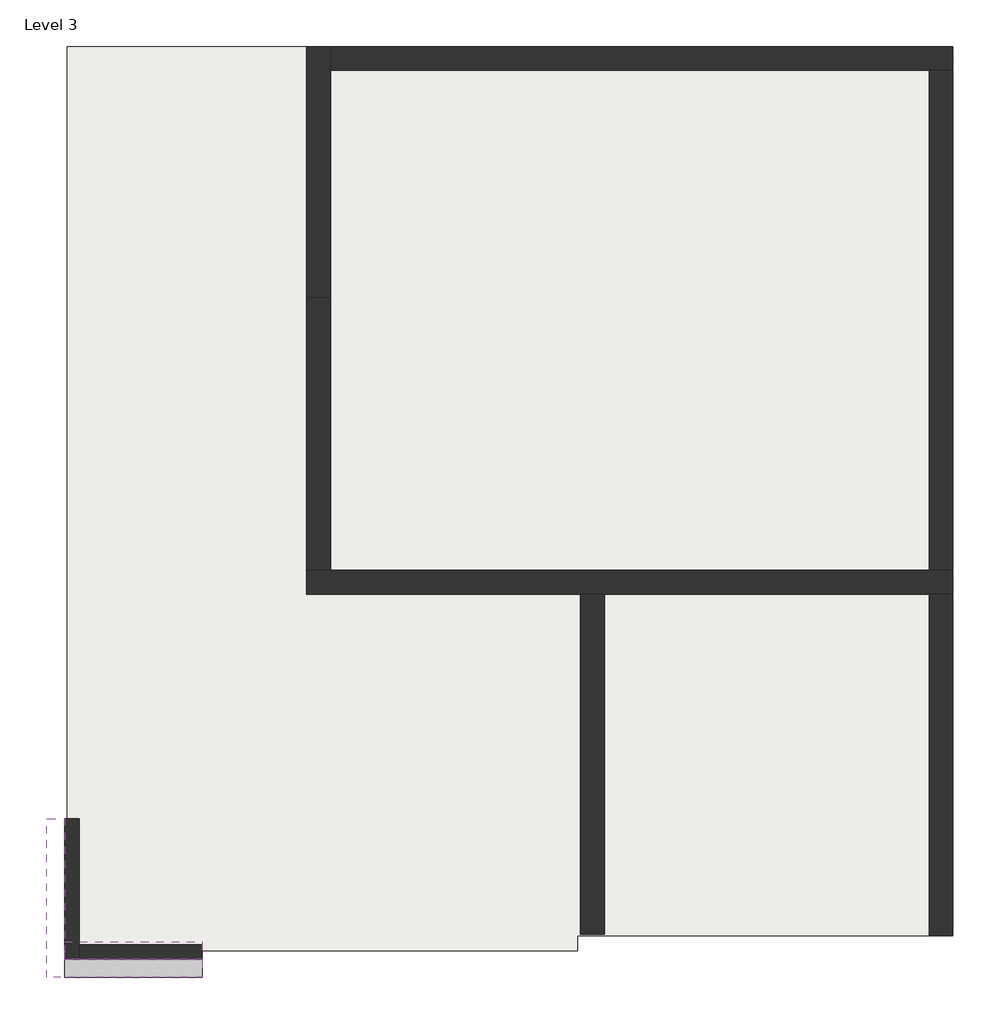
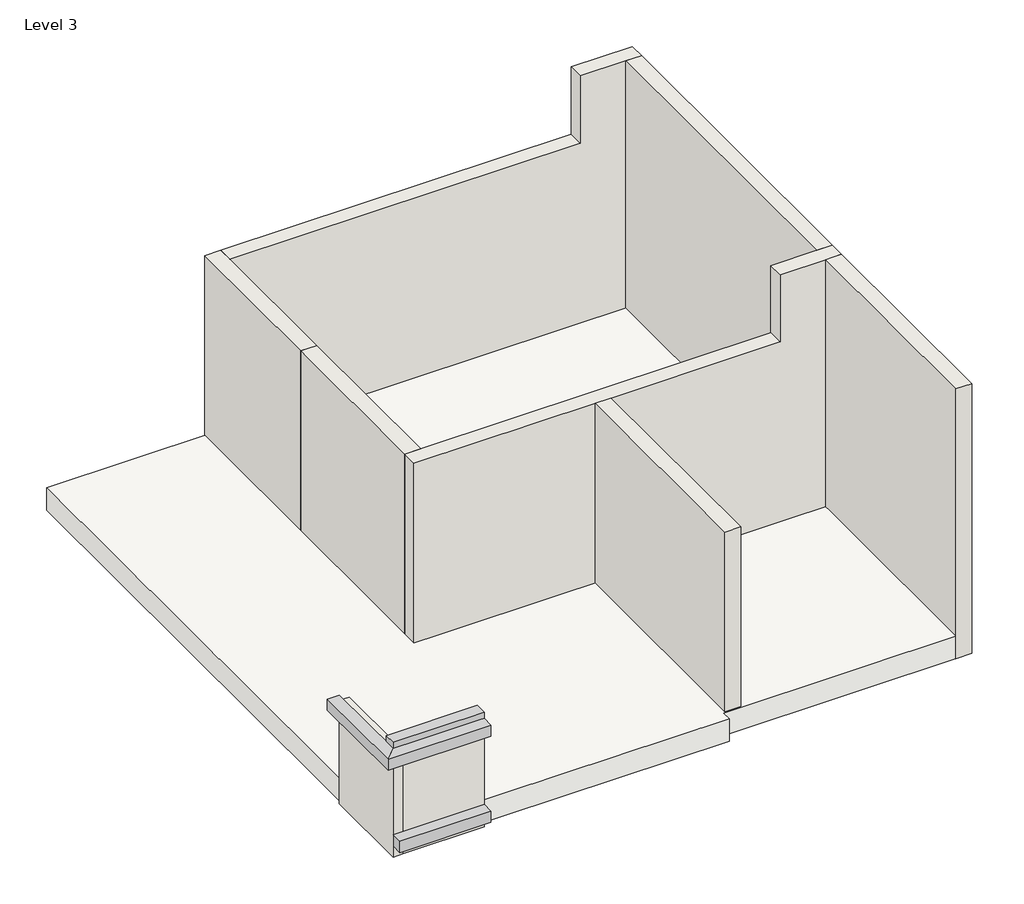
# One storey, incomplete: 9 walls, 3 proxies, 1 roof.
"""IFC4 building model written with IfcOpenShell, lengths in millimetres."""

from ifc_helpers import new_model, si_unit, frame, origin, place, context, project, spatial, polyline, outline, extrude, faceted_brep, element, save

model = new_model("IFC4")

# Units and contexts
model_context = context("Model", 3, world=origin())
ifc_project = project(units=[si_unit("LENGTHUNIT", "METRE", prefix="MILLI")], contexts=[model_context])

# Site, building, storey
site = spatial("IfcSite", under=ifc_project)
building = spatial("IfcBuilding", under=site)
storey = spatial("IfcBuildingStorey", under=building, Name="Level 3", Elevation=7315.2)

# Proxies
placement = place(None, origin())
element("IfcBuildingElementProxy", 1, Name="Cornice", ObjectType="Cornice", at=placement, inside=storey, context=model_context, shape_type="SweptSolid", body=[
    extrude(outline(polyline([(-7893.9125658, 3843.7483979), (-7741.5125658, 3996.1483979), (-6573.1125658, 3996.1483979), (-6573.1125658, 3843.7483979), (-7893.9125658, 3843.7483979)])), frame((0.0, 0.0, 8636.0), z_axis=(0.0, 0.0, 1.0), x_axis=(1.0, 0.0, 0.0)), (0.0, 0.0, 1.0), 152.4),
    extrude(outline(polyline([(-7893.9125658, 5189.9483979), (-7741.5125658, 5189.9483979), (-7741.5125658, 3996.1483979), (-7893.9125658, 3843.7483979), (-7893.9125658, 5189.9483979)])), frame((0.0, 0.0, 8636.0), z_axis=(0.0, 0.0, 1.0), x_axis=(1.0, 0.0, 0.0)), (0.0, 0.0, 1.0), 152.4),
])
element("IfcBuildingElementProxy", 2, Name="Cornice", ObjectType="Cornice", at=placement, inside=storey, context=model_context, shape_type="SweptSolid", body=[
    extrude(outline(polyline([(-7741.5125658, 3843.7483979), (-7741.5125658, 3996.1483979), (-6573.1125658, 3996.1483979), (-6573.1125658, 3843.7483979), (-7741.5125658, 3843.7483979)])), frame((0.0, 0.0, 7467.6), z_axis=(0.0, 0.0, 1.0), x_axis=(1.0, 0.0, 0.0)), (0.0, 0.0, 1.0), 152.4),
])
element("IfcBuildingElementProxy", 3, Name="Reveal", ObjectType="Reveal", at=placement, inside=storey, context=model_context, shape_type="SweptSolid", body=[
    extrude(outline(polyline([(-7741.5125658, 3996.1483979), (-7741.5125658, 4148.5483979), (-6573.1125658, 4148.5483979), (-6573.1125658, 3996.1483979), (-7741.5125658, 3996.1483979)])), frame((0.0, 0.0, 8717.2601563), z_axis=(0.0, 0.0, 1.0), x_axis=(1.0, 0.0, 0.0)), (0.0, 0.0, 1.0), 152.4),
])

# Roof
element("IfcRoof", 4, ObjectType="Generic - 12\"", at=placement, inside=storey, context=model_context, shape_type="SweptSolid", body=[
    extrude(outline(polyline([(-7716.1125658, 11743.1483979), (-197.7125658, 11743.1483979), (-197.7125658, 4199.3483979), (-3385.4125658, 4199.3483979), (-3385.4125658, 4072.3483979), (-7716.1125658, 4072.3483979), (-7716.1125658, 11743.1483979)])), frame((0.0, 0.0, 7315.2), z_axis=(0.0, 0.0, 1.0), x_axis=(1.0, 0.0, 0.0)), (0.0, 0.0, 1.0), 304.8),
])

# Walls
element("IfcWall", 5, ObjectType="Generic - 5\"", at=placement, inside=storey, context=model_context, shape_type="Brep", body=[
    faceted_brep([(-7741.5125658, 5189.9483979, 7315.2), (-7741.5125658, 3996.1483979, 7315.2), (-7741.5125658, 3996.1483979, 8636.0), (-7741.5125658, 3996.1483979, 8717.2601563), (-7741.5125658, 5189.9483979, 8717.2601563), (-7741.5125658, 5189.9483979, 8636.0), (-7614.5125658, 3996.1483979, 7315.2), (-7614.5125658, 4123.1483979, 7315.2), (-7614.5125658, 5189.9483979, 7315.2), (-7614.5125658, 5189.9483979, 8717.2601563), (-7614.5125658, 4123.1483979, 8717.2601563), (-7614.5125658, 3996.1483979, 8717.2601563), (-7614.5125658, 3996.1483979, 8636.0)], [[[0, 1, 2, 3, 4, 5]], [[6, 7, 8, 9, 10, 11, 12]], [[1, 0, 8, 7, 6]], [[4, 3, 11, 10, 9]], [[9, 8, 0, 5, 4]], [[1, 6, 12, 11, 3, 2]]]),
])
element("IfcWall", 6, ObjectType="Generic - 5\"", at=placement, inside=storey, context=model_context, shape_type="Brep", body=[
    faceted_brep([(-7614.5125658, 3996.1483979, 7315.2), (-6573.1125658, 3996.1483979, 7315.2), (-6573.1125658, 3996.1483979, 8636.0), (-6573.1125658, 3996.1483979, 8717.2601563), (-7614.5125658, 3996.1483979, 8717.2601563), (-7614.5125658, 3996.1483979, 8636.0), (-6573.1125658, 4123.1483979, 7315.2), (-7614.5125658, 4123.1483979, 7315.2), (-7614.5125658, 4123.1483979, 8717.2601563), (-6573.1125658, 4123.1483979, 8717.2601563)], [[[0, 1, 2, 3, 4, 5]], [[6, 7, 8, 9]], [[1, 0, 7, 6]], [[6, 9, 3, 2, 1]], [[4, 3, 9, 8]], [[4, 8, 7, 0, 5]]]),
])
element("IfcWall", 7, ObjectType="Generic - 8\"", at=placement, inside=storey, context=model_context, shape_type="Brep", body=[
    faceted_brep([(-197.7125658, 7298.1483979, 7315.2), (-400.9125658, 7298.1483979, 7315.2), (-5480.9125658, 7298.1483979, 7315.2), (-5684.1125658, 7298.1483979, 7315.2), (-5684.1125658, 7298.1483979, 10058.4), (-5480.9125658, 7298.1483979, 10058.4), (-985.1125658, 7298.1483979, 10058.4), (-985.1125658, 7298.1483979, 10972.8), (-400.9125658, 7298.1483979, 10972.8), (-197.7125658, 7298.1483979, 10972.8), (-197.7125658, 7094.9483979, 7315.2), (-197.7125658, 7094.9483979, 10972.8), (-400.9125658, 7094.9483979, 10972.8), (-985.1125658, 7094.9483979, 10972.8), (-985.1125658, 7094.9483979, 10058.4), (-3156.8125658, 7094.9483979, 10058.4), (-3360.0125658, 7094.9483979, 10058.4), (-5684.1125658, 7094.9483979, 10058.4), (-5684.1125658, 7094.9483979, 7315.2), (-3360.0125658, 7094.9483979, 7315.2), (-3156.8125658, 7094.9483979, 7315.2), (-400.9125658, 7094.9483979, 7315.2)], [[[0, 1, 2, 3, 4, 5, 6, 7, 8, 9]], [[10, 11, 12, 13, 14, 15, 16, 17, 18, 19, 20, 21]], [[3, 2, 1, 0, 10, 21, 20, 19, 18]], [[4, 3, 18, 17]], [[0, 9, 11, 10]], [[9, 8, 7, 13, 12, 11]], [[13, 7, 6, 14]], [[6, 5, 4, 17, 16, 15, 14]]]),
])
element("IfcWall", 8, ObjectType="Generic - 8\"", at=placement, inside=storey, context=model_context, shape_type="SweptSolid", body=[
    extrude(outline(polyline([(-5480.9125658, 9609.5483979), (-5480.9125658, 7298.1483979), (-5684.1125658, 7298.1483979), (-5684.1125658, 9609.5483979), (-5480.9125658, 9609.5483979)])), frame((0.0, 0.0, 7315.2), z_axis=(0.0, 0.0, 1.0), x_axis=(1.0, 0.0, 0.0)), (0.0, 0.0, 1.0), 2743.2),
])
element("IfcWall", 9, ObjectType="Generic - 8\"", at=placement, inside=storey, context=model_context, shape_type="Brep", body=[
    faceted_brep([(-5480.9125658, 9609.5483979, 7315.2), (-5480.9125658, 11539.9483979, 7315.2), (-5480.9125658, 11743.1483979, 7315.2), (-5480.9125658, 11743.1483979, 10058.4), (-5480.9125658, 11539.9483979, 10058.4), (-5480.9125658, 9609.5483979, 10058.4), (-5684.1125658, 9609.5483979, 7315.2), (-5684.1125658, 9609.5483979, 10058.4), (-5684.1125658, 11743.1483979, 10058.4), (-5684.1125658, 11743.1483979, 7315.2)], [[[0, 1, 2, 3, 4, 5]], [[6, 7, 8, 9]], [[2, 1, 0, 6, 9]], [[0, 5, 7, 6]], [[3, 2, 9, 8]], [[5, 4, 3, 8, 7]]]),
])
element("IfcWall", 10, ObjectType="Generic - 8\"", at=placement, inside=storey, context=model_context, shape_type="Brep", body=[
    faceted_brep([(-5480.9125658, 11539.9483979, 7315.2), (-400.9125658, 11539.9483979, 7315.2), (-197.7125658, 11539.9483979, 7315.2), (-197.7125658, 11539.9483979, 10972.8), (-400.9125658, 11539.9483979, 10972.8), (-985.1125658, 11539.9483979, 10972.8), (-985.1125658, 11539.9483979, 10058.4), (-5480.9125658, 11539.9483979, 10058.4), (-5480.9125658, 11743.1483979, 7315.2), (-5480.9125658, 11743.1483979, 10058.4), (-985.1125658, 11743.1483979, 10058.4), (-985.1125658, 11743.1483979, 10972.8), (-197.7125658, 11743.1483979, 10972.8), (-197.7125658, 11743.1483979, 7315.2)], [[[0, 1, 2, 3, 4, 5, 6, 7]], [[8, 9, 10, 11, 12, 13]], [[2, 1, 0, 8, 13]], [[0, 7, 9, 8]], [[5, 4, 3, 12, 11]], [[5, 11, 10, 6]], [[7, 6, 10, 9]], [[2, 13, 12, 3]]]),
])
element("IfcWall", 11, ObjectType="Generic - 8\"", at=placement, inside=storey, context=model_context, shape_type="SweptSolid", body=[
    extrude(outline(polyline([(-400.9125658, 7298.1483979), (-400.9125658, 11539.9483979), (-197.7125658, 11539.9483979), (-197.7125658, 7298.1483979), (-400.9125658, 7298.1483979)])), frame((0.0, 0.0, 7315.2), z_axis=(0.0, 0.0, 1.0), x_axis=(1.0, 0.0, 0.0)), (0.0, 0.0, 1.0), 3657.6),
])
element("IfcWall", 12, ObjectType="Generic - 8\"", at=placement, inside=storey, context=model_context, shape_type="SweptSolid", body=[
    extrude(outline(polyline([(-3360.0125658, 4212.0483979), (-3360.0125658, 7094.9483979), (-3156.8125658, 7094.9483979), (-3156.8125658, 4212.0483979), (-3360.0125658, 4212.0483979)])), frame((0.0, 0.0, 7315.2), z_axis=(0.0, 0.0, 1.0), x_axis=(1.0, 0.0, 0.0)), (0.0, 0.0, 1.0), 2743.2),
])
element("IfcWall", 13, ObjectType="Generic - 8\"", at=placement, inside=storey, context=model_context, shape_type="SweptSolid", body=[
    extrude(outline(polyline([(-400.9125658, 4199.3483979), (-400.9125658, 7094.9483979), (-197.7125658, 7094.9483979), (-197.7125658, 4199.3483979), (-400.9125658, 4199.3483979)])), frame((0.0, 0.0, 7315.2), z_axis=(0.0, 0.0, 1.0), x_axis=(1.0, 0.0, 0.0)), (0.0, 0.0, 1.0), 3657.6),
])

save(model, "model.ifc")

# Revit data of these elements
# Type "Generic - 12\""
#   Assembly Code = "B1020"
#   Layers, outside or top first: 1' - 0" no material (function 1)
# Type "Generic - 5\""
#   Assembly Code = "B2010"
#   Layers, outside or top first: 0' - 5" no material (function 1)
# Type "Generic - 8\""
#   Assembly Code = "B2010"
#   Layers, outside or top first: 0' - 8" no material (function 1)
# Elements 1, 2 (IfcBuildingElementProxy, "Cornice")
#   Phase Created = New Construction
#   Materials on its faces: "Default Wall"
# Element 4 (IfcRoof, "Generic - 12\"")
#   built-in parameter 1001705 = 25 (stored number, unit not read)
#   built-in parameter 1001710 = 33615
#   Phase Created = New Construction
#   Materials on its faces: "Default Roof"
# Elements 5, 6 (IfcWall, "Generic - 5\"")
#   Top Offset = -7' - 4 205/256"
#   Base Offset = 0' - 0"
#   wall height = 4' - 7 51/256"
#   Phase Created = New Construction
#   Base Constraint = Level 3
#   Top Constraint = Level 4
#   Materials on its faces: "Default Wall"
# Elements 7, 8, 9, 10, 11, 12, 13 (IfcWall, "Generic - 8\"")
#   Top Offset = 0' - 0"
#   Base Offset = 0' - 0"
#   Unconnected Height = 12' - 0"
#   wall height = 12' - 0"
#   Phase Created = New Construction
#   Base Constraint = Level 3
#   Materials on its faces: "Default Wall"
# Materials
#   "Default Wall": colour RGB 128 128 128, transparency 0
#   "Default Roof": colour RGB 88 101 114, transparency 0
